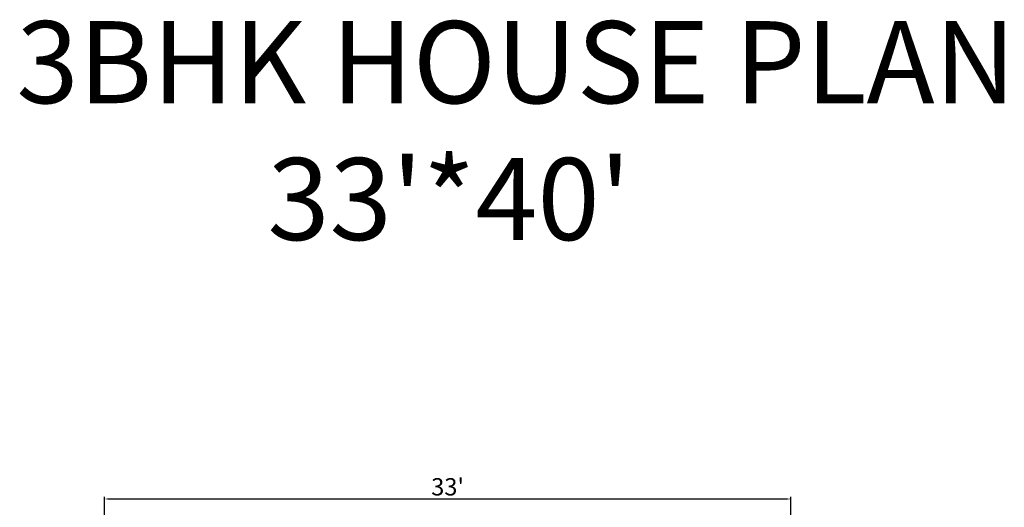
# Model space of a CAD drawing. Units: inches. Extents: x 1822 to 2392, y 2066 to 2908.
# Tile 4 of 4: x 1823 to 2392, y 2627 to 2908. Entities that reach past the tile are written whole.
import ezdxf

# ---------------------------------------------------------------- set-up
doc = ezdxf.new("R2010")
doc.units = ezdxf.units.IN
doc.layers.add('A-ANNO-DIMS', color=2, linetype='Continuous', lineweight=18)
doc.layers.add('TEXT', color=83, linetype='Continuous', lineweight=25)
doc.styles.get("Standard").update_dxf_attribs({"font": 'arial.ttf'})
doc.dimstyles.new('ISO-25', dxfattribs={"dimtxt": 10, "dimasz": 2.5, "dimexe": 1.25, "dimexo": 0.625, "dimtad": 1, "dimdec": 0, "dimlunit": 4, "dimtxsty": 'Standard', "dimcen": 2.5, "dimadec": 0, "dimazin": 0, "dimtfac": 1, "dimtdec": 0, "dimtmove": 0, "dimatfit": 3, "dimfxl": 1, "dimarcsym": 0})

# ---------------------------------------------------------------- blocks, each defined once
blk = doc.blocks.new('*D5')
at = {"layer": 'A-ANNO-DIMS', "color": 0, "lineweight": -2, "transparency": 16777216}
for p, q in [((1872.41, 2584.74), (1872.41, 2632.85)), ((1874.91, 2631.6), (2265.91, 2631.6)), ((2268.41, 2584.74), (2268.41, 2632.85))]:
    blk.add_line(p, q, dxfattribs=at)
at = {"layer": 'A-ANNO-DIMS', "color": 0, "transparency": 16777216}
for points in [[(1874.91, 2632.01), (1874.91, 2631.18), (1872.41, 2631.6)], [(2265.91, 2632.01), (2265.91, 2631.18), (2268.41, 2631.6)]]:
    blk.add_solid(points, dxfattribs=at)
at = {"layer": 'Defpoints', "color": 0, "transparency": 16777216}
for p in [(2268.41, 2631.6), (1872.41, 2584.12), (2268.41, 2584.12)]:
    blk.add_point(p, dxfattribs=at)
at = {"layer": 'A-ANNO-DIMS', "color": 0, "transparency": 16777216, "insert": (2070.41, 2637.33), "char_height": 10, "attachment_point": 5}
blk.add_mtext("33'", dxfattribs=at)

msp = doc.modelspace()

# ---------------------------------------------------------------- texts
at = {"layer": 'TEXT', "insert": (1821.59, 2907.5), "char_height": 47.3994, "attachment_point": 1}
msp.add_mtext_dynamic_manual_height_columns("3BHK HOUSE PLAN\\P          33'*40'", width=6784.8941, gutter_width=237, heights=[0], dxfattribs=at)

# ---------------------------------------------------------------- dimensions: what is measured, and where the dimension line sits
at = {"layer": 'A-ANNO-DIMS'}
dim = msp.add_linear_dim(base=(2268.41, 2631.6), p1=(1872.41, 2584.12), p2=(2268.41, 2584.12), dimstyle='ISO-25', override={"dimclrd": 0, "dimclre": 0, "dimclrt": 0}, dxfattribs=at)
dim.commit()
dim.dimension.update_dxf_attribs({"geometry": '*D5', "text_midpoint": (2070.41, 2637.33)})

doc.saveas('drawing.dxf')
